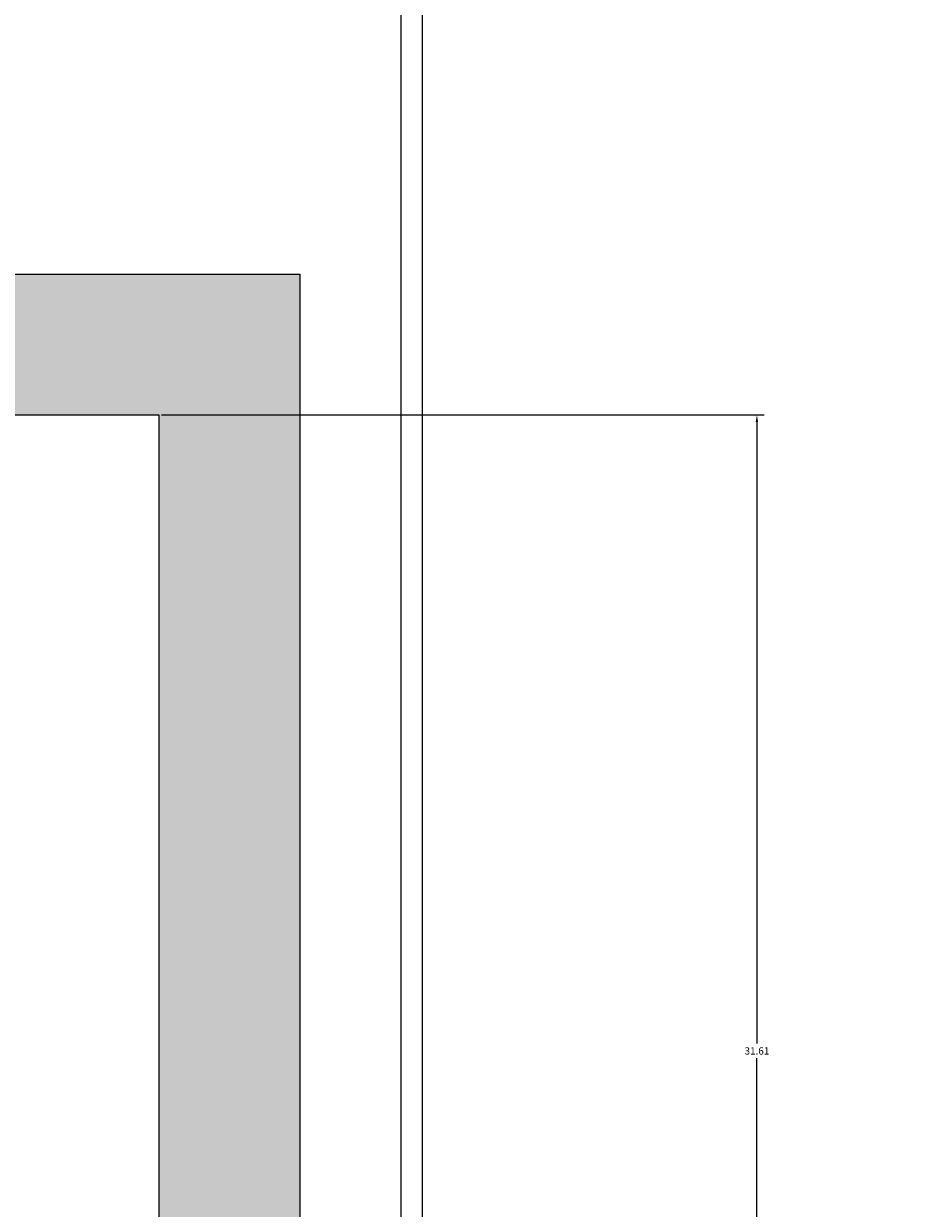
# Model space of a CAD drawing. Units: millimetres. Extents: x -11 to 280, y -4 to 208.
# Tile 38 of 55: x 222 to 244, y 55 to 85. Entities that reach past the tile are written whole.
import ezdxf

# ---------------------------------------------------------------- set-up
doc = ezdxf.new("R2010")
doc.units = ezdxf.units.MM
doc.layers.add('M-DIMS', color=2, linetype='Continuous', lineweight=18)
doc.layers.add('M-HYDR-PRES', color=7, linetype='Continuous', lineweight=25)
doc.layers.add('M-HYDR-PRES-PATT', color=240, linetype='Continuous', lineweight=13, true_color=0xed1f24)
doc.styles.get("Standard").update_dxf_attribs({"font": 'arial.ttf'})
doc.dimstyles.get("Standard").update_dxf_attribs({"dimtxt": 0.18, "dimasz": 0.18, "dimexe": 0.18, "dimexo": 0.0625, "dimgap": 0.09, "dimtad": 0, "dimtih": 1, "dimtoh": 1, "dimdec": 4, "dimzin": 0, "dimdsep": 46, "dimtxsty": 'Standard', "dimcen": 0.09, "dimadec": 0, "dimazin": 0, "dimtfac": 1, "dimtdec": 4, "dimtofl": 0, "dimtmove": 0, "dimatfit": 3, "dimfxl": 1, "dimtolj": 1, "dimtzin": 0, "dimarcsym": 0})

# ---------------------------------------------------------------- blocks, each defined once
blk = doc.blocks.new('*D4')
at = {"layer": 'Defpoints', "color": 0, "transparency": 16777216}
for p in [(4.763, 84.426), (266.035, 51.733), (266.035, -3.415)]:
    blk.add_point(p, dxfattribs=at)
at = {"layer": 'M-DIMS', "color": 0, "lineweight": -2, "transparency": 16777216}
for p, q in [((4.763, 84.364), (4.763, -3.595)), ((266.035, 51.67), (266.035, -3.595)), ((4.943, -3.415), (134.934, -3.415)), ((265.855, -3.415), (135.864, -3.415))]:
    blk.add_line(p, q, dxfattribs=at)
at = {"layer": 'M-DIMS', "color": 0, "transparency": 16777216}
for points in [[(4.943, -3.385), (4.943, -3.445), (4.763, -3.415)], [(265.855, -3.385), (265.855, -3.445), (266.035, -3.415)]]:
    blk.add_solid(points, dxfattribs=at)
at = {"layer": 'M-DIMS', "color": 0, "transparency": 16777216, "insert": (135.399, -3.415), "char_height": 0.18, "attachment_point": 5}
blk.add_mtext('\\A1;261.27', dxfattribs=at)
blk = doc.blocks.new('*D5')
at = {"layer": 'Defpoints', "color": 0, "transparency": 16777216}
for p in [(24.759, 192.645), (-10.087, 11.435), (261.686, 11.435)]:
    blk.add_point(p, dxfattribs=at)
at = {"layer": 'M-DIMS', "color": 0, "lineweight": -2, "transparency": 16777216}
for p, q in [((24.696, 192.645), (-10.267, 192.645)), ((-10.087, 192.465), (-10.087, 102.222)), ((-10.087, 11.615), (-10.087, 101.858)), ((261.624, 11.435), (-10.267, 11.435))]:
    blk.add_line(p, q, dxfattribs=at)
at = {"layer": 'M-DIMS', "color": 0, "transparency": 16777216}
for points in [[(-10.117, 192.465), (-10.057, 192.465), (-10.087, 192.645)], [(-10.117, 11.615), (-10.057, 11.615), (-10.087, 11.435)]]:
    blk.add_solid(points, dxfattribs=at)
at = {"layer": 'M-DIMS', "color": 0, "transparency": 16777216, "insert": (-10.087, 102.04), "char_height": 0.18, "attachment_point": 5}
blk.add_mtext('\\A1;181.2', dxfattribs=at)
blk = doc.blocks.new('*D13')
at = {"layer": 'Defpoints', "color": 0, "transparency": 16777216}
for p in [(191.774, 105.314), (232.2, 105.314), (232.2, -3.415)]:
    blk.add_point(p, dxfattribs=at)
at = {"layer": 'M-DIMS', "color": 0, "lineweight": -2, "transparency": 16777216}
for p, q in [((191.774, 105.252), (191.774, -3.595)), ((232.2, 105.252), (232.2, -3.595)), ((191.954, -3.415), (211.52, -3.415)), ((232.02, -3.415), (212.454, -3.415))]:
    blk.add_line(p, q, dxfattribs=at)
at = {"layer": 'M-DIMS', "color": 0, "transparency": 16777216}
for points in [[(191.954, -3.385), (191.954, -3.445), (191.774, -3.415)], [(232.02, -3.385), (232.02, -3.445), (232.2, -3.415)]]:
    blk.add_solid(points, dxfattribs=at)
at = {"layer": 'M-DIMS', "color": 0, "transparency": 16777216, "insert": (211.987, -3.415), "char_height": 0.18, "attachment_point": 5}
blk.add_mtext('\\A1;40.426', dxfattribs=at)
blk = doc.blocks.new('*D19')
at = {"layer": 'Defpoints', "color": 0, "transparency": 16777216}
for p in [(225.662, 75.21), (225.662, 43.599), (240.512, 43.599)]:
    blk.add_point(p, dxfattribs=at)
at = {"layer": 'M-DIMS', "color": 0, "lineweight": -2, "transparency": 16777216}
for p, q in [((225.724, 75.21), (240.692, 75.21)), ((240.512, 75.03), (240.512, 59.586)), ((240.512, 43.779), (240.512, 59.222)), ((225.724, 43.599), (240.692, 43.599))]:
    blk.add_line(p, q, dxfattribs=at)
at = {"layer": 'M-DIMS', "color": 0, "transparency": 16777216}
for points in [[(240.482, 75.03), (240.542, 75.03), (240.512, 75.21)], [(240.482, 43.779), (240.542, 43.779), (240.512, 43.599)]]:
    blk.add_solid(points, dxfattribs=at)
at = {"layer": 'M-DIMS', "color": 0, "transparency": 16777216, "insert": (240.512, 59.404), "char_height": 0.18, "attachment_point": 5}
blk.add_mtext('\\A1;31.61', dxfattribs=at)
blk = doc.blocks.new('*D20')
at = {"layer": 'Defpoints', "color": 0, "transparency": 16777216}
for p in [(231.68, 207.495), (151.022, 43.599), (231.68, 43.599)]:
    blk.add_point(p, dxfattribs=at)
at = {"layer": 'M-DIMS', "color": 0, "lineweight": -2, "transparency": 16777216}
for p, q in [((151.022, 43.662), (151.022, 207.675)), ((231.68, 43.662), (231.68, 207.675)), ((151.202, 207.495), (190.957, 207.495)), ((231.5, 207.495), (191.745, 207.495))]:
    blk.add_line(p, q, dxfattribs=at)
at = {"layer": 'M-DIMS', "color": 0, "transparency": 16777216}
for points in [[(151.202, 207.525), (151.202, 207.465), (151.022, 207.495)], [(231.5, 207.525), (231.5, 207.465), (231.68, 207.495)]]:
    blk.add_solid(points, dxfattribs=at)
at = {"layer": 'M-DIMS', "color": 0, "transparency": 16777216, "insert": (191.351, 207.495), "char_height": 0.18, "attachment_point": 5}
blk.add_mtext('\\A1;80.66', dxfattribs=at)
blk = doc.blocks.new('*D22')
at = {"layer": 'Defpoints', "color": 0, "transparency": 16777216}
for p in [(259.871, 207.495), (231.68, 34.723), (259.871, 34.723)]:
    blk.add_point(p, dxfattribs=at)
at = {"layer": 'M-DIMS', "color": 0, "lineweight": -2, "transparency": 16777216}
for p, q in [((231.68, 34.785), (231.68, 207.675)), ((259.871, 34.785), (259.871, 207.675)), ((231.86, 207.495), (245.38, 207.495)), ((259.691, 207.495), (246.171, 207.495))]:
    blk.add_line(p, q, dxfattribs=at)
at = {"layer": 'M-DIMS', "color": 0, "transparency": 16777216}
for points in [[(231.86, 207.525), (231.86, 207.465), (231.68, 207.495)], [(259.691, 207.525), (259.691, 207.465), (259.871, 207.495)]]:
    blk.add_solid(points, dxfattribs=at)
at = {"layer": 'M-DIMS', "color": 0, "transparency": 16777216, "insert": (245.776, 207.495), "char_height": 0.18, "attachment_point": 5}
blk.add_mtext('\\A1;28.19', dxfattribs=at)

msp = doc.modelspace()

# ---------------------------------------------------------------- hatches: boundary and pattern name
at = {"layer": 'M-HYDR-PRES-PATT'}
h = msp.add_hatch(color=256, dxfattribs=at)
h.set_gradient(color1=(237, 31, 36), color2=(237, 31, 36), tint=1)
h.paths.add_polyline_path([(232.2, 133.1228), (228.7, 133.1228), (228.7, 108.8141), (102.7646, 108.8141), (102.7646, 105.3141), (232.2, 105.3141)])
h.paths.add_polyline_path([(128.8433, 105.3141), (125.3433, 105.3141), (125.3433, 91.7099, 1), (128.8433, 91.7099)])
h.paths.add_polyline_path([(229.1617, 78.7098), (196.7745, 78.7098, -0.4142136), (191.7745, 83.7098), (191.7745, 105.3141), (188.2745, 105.3141), (188.2745, 80.2098, 0.4142136), (193.2745, 75.2098), (225.6617, 75.2098), (225.6617, 43.5991), (229.1617, 43.5991)])
h.paths.add_polyline_path([(102.7646, 110.3704), (95.5776, 110.3704), (95.5776, 103.9022), (102.7646, 103.9022)])
h.paths.add_polyline_path([(100.7059, 107.2502), (99.1711, 106.3641), (99.1711, 106.8641), (97.1711, 106.8641), (97.1711, 107.6363), (99.1711, 107.6363), (99.1711, 108.1363)], flags=16)
h.paths.add_polyline_path([(234.6119, 138.4081), (226.5106, 138.4081), (226.5106, 133.1228), (234.6119, 133.1228)])
h.paths.add_polyline_path([(231.1963, 135.7055), (230.2965, 134.1786), (229.4241, 135.7213), (229.9241, 135.7168), (229.9418, 137.7167), (230.7141, 137.7099), (230.6963, 135.71)], flags=16)

# ---------------------------------------------------------------- linework, layer by layer
at = {"layer": 'M-HYDR-PRES'}
for points in [[(188.2745, 105.3141), (188.2745, 80.2098, 0.4142136), (193.2745, 75.2098), (225.6617, 75.2098), (225.6617, 43.5991)], [(191.7745, 105.3141), (191.7745, 83.7098, 0.4142136), (196.7745, 78.7098), (229.1617, 78.7098), (229.1617, 43.5991)]]:
    msp.add_lwpolyline(points, format="xyb", dxfattribs=at)

# ---------------------------------------------------------------- dimensions: what is measured, and where the dimension line sits
at = {"layer": 'M-DIMS'}
for base, p1, p2, override, picture, middle in [((231.6803, 207.495), (151.0217, 43.5991), (231.6803, 43.5991), {"dimdec": 2, "dimlfac": 1, "dimrnd": 0, "dimzin": 0, "dimdsep": 46, "dimlunit": 2}, '*D20', (191.351, 207.495)), ((259.871, 207.495), (231.6803, 34.7226), (259.871, 34.7226), {"dimdec": 2, "dimlfac": 1, "dimrnd": 0, "dimzin": 0, "dimdsep": 46, "dimlunit": 2}, '*D22', (245.7757, 207.495)), ((232.20002, -3.41542), (191.77448, 105.31407), (232.20002, 105.31407), {"dimdec": 3, "dimlfac": 1, "dimrnd": 0, "dimzin": 0, "dimdsep": 46, "dimlunit": 2}, '*D13', (211.98725, -3.41542)), ((266.0352, -3.4154), (4.7635, 84.4261), (266.0352, 51.7328), {"dimdec": 2, "dimlfac": 1, "dimrnd": 0, "dimzin": 0, "dimdsep": 46, "dimlunit": 2}, '*D4', (135.3993, -3.4154))]:
    dim = msp.add_linear_dim(base=base, p1=p1, p2=p2, dimstyle='Standard', override=override, dxfattribs=at)
    dim.commit()
    dim.dimension.update_dxf_attribs({"geometry": picture, "text_midpoint": middle})
for base, p1, p2, angle, override, picture, middle in [((-10.0865, 11.4346), (24.7588, 192.645), (261.6863, 11.4346), 90, {"dimdec": 1, "dimlfac": 1, "dimrnd": 0, "dimzin": 0, "dimdsep": 46, "dimlunit": 2}, '*D5', (-10.0865, 102.0398)), ((240.5117, 43.5991), (225.6617, 75.2098), (225.6617, 43.5991), 270, {"dimdec": 2, "dimlfac": 1, "dimrnd": 0, "dimzin": 0, "dimdsep": 46, "dimlunit": 2}, '*D19', (240.5117, 59.4044))]:
    dim = msp.add_linear_dim(base=base, p1=p1, p2=p2, angle=angle, dimstyle='Standard', override=override, dxfattribs=at)
    dim.commit()
    dim.dimension.update_dxf_attribs({"geometry": picture, "text_midpoint": middle})

doc.saveas('drawing.dxf')
